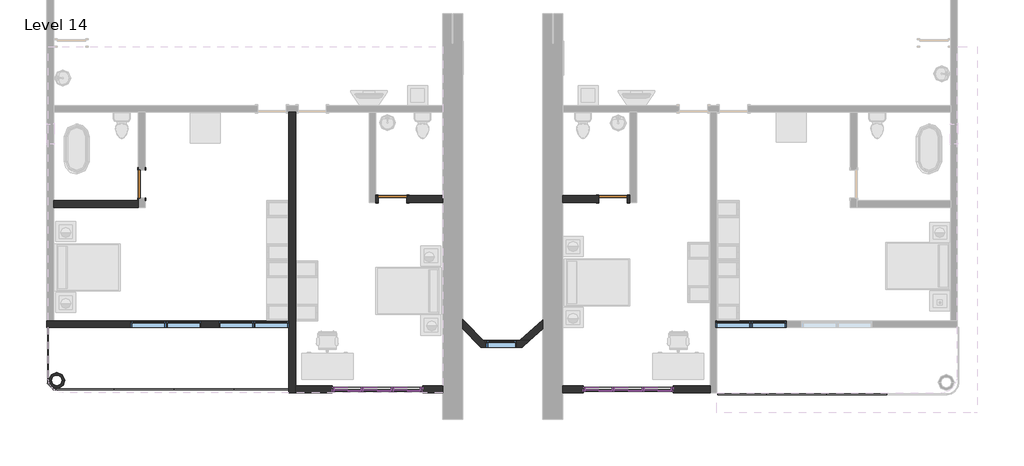
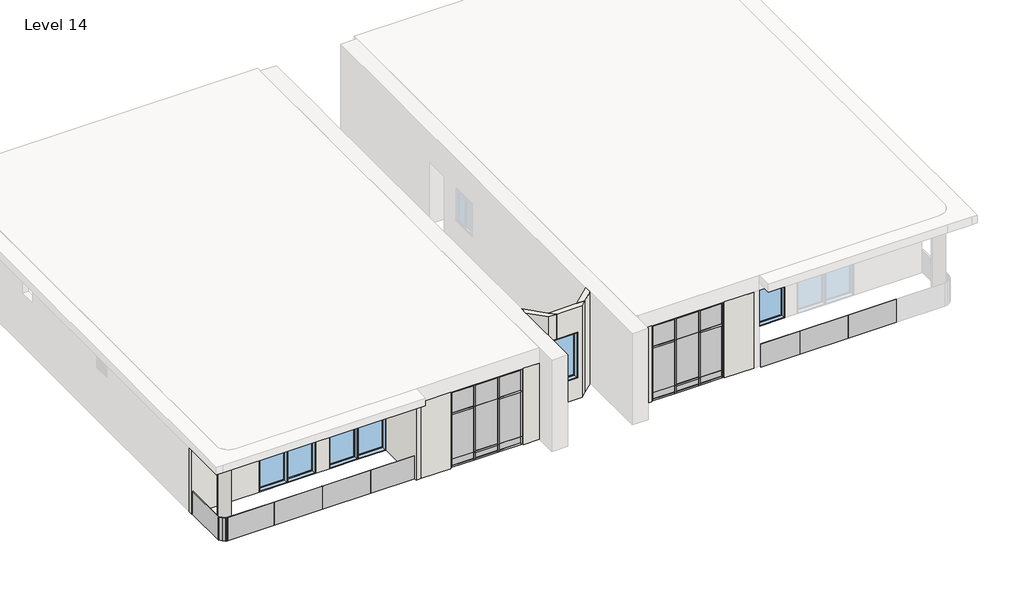
# One storey, part 1 of 3: 42 members, 30 plates, 14 walls, 7 windows, 3 doors.
"""IFC4 building model written with IfcOpenShell, lengths in millimetres."""

from ifc_helpers import new_model, si_unit, point, frame, frame_2d, origin, place, context, project, spatial, polyline, circle_curve, trimmed, segment, composite_curve, outline, extrude, faceted_brep, transform, mapped, element, save
from components import door_2703ae13, door_10fd3a06, member_c17f1be2, member_ad567e07, member_d2e7e466, member_7db1855a, member_75d1e245, member_d60e8053, member_3c3dc66a, member_2fae0574, member_410c6227, member_73c23c35, system_panel_glazed_38d54ecf, system_panel_glazed_fbb6c980, system_panel_glazed_4137532c, system_panel_glazed_6230de04, system_panel_glazed_a79f7f85, system_panel_glazed_9a5ea490, system_panel_glazed_95be5de7, system_panel_glazed_1e00a1c5, system_panel_glazed_ffe51582, system_panel_glazed_8f95e3f6, system_panel_glazed_836907cd, system_panel_glazed_688a65a2, system_panel_glazed_c1a1c740, system_panel_glazed_22bcd51f, window_9a779fa2, window_1a213a25

model = new_model("IFC4")

# Units and contexts
model_context = context("Model", 3, world=origin())
ifc_project = project(units=[si_unit("LENGTHUNIT", "METRE", prefix="MILLI")], contexts=[model_context])

# Site, building, storey
site = spatial("IfcSite", under=ifc_project)
building = spatial("IfcBuilding", under=site)
storey = spatial("IfcBuildingStorey", under=building, Name="Level 14", Elevation=47548.8)

# Doors
placement = place(None, origin())
door_shape = door_2703ae13(model_context)
element("IfcDoor", 1, ObjectType="Door-Single-Panel.0001 : 34\" x 80\"", at=placement, inside=storey, context=model_context, shape_type="MappedRepresentation", body=[
    mapped(door_shape, transform((-15765.9987704, -441.9241442, 47548.8), x_axis=(0.0, -1.0, 0.0), y_axis=(1.0, 0.0, 0.0), z_axis=(0.0, 0.0, 1.0))),
])
element("IfcDoor", 2, ObjectType="Door-Single-Panel.0001 : 34\" x 80\"", at=placement, inside=storey, context=model_context, shape_type="MappedRepresentation", body=[
    mapped(door_shape, transform((-8145.9987704, -899.1241442, 47548.8), x_axis=(-1.0, 0.0, 0.0), y_axis=(0.0, -1.0, 0.0), z_axis=(0.0, 0.0, 1.0))),
])
door_2_shape = door_10fd3a06(model_context)
element("IfcDoor", 3, ObjectType="Door-Single-Panel.0001 : 34\" x 80\"", at=placement, inside=storey, context=model_context, shape_type="MappedRepresentation", body=[
    mapped(door_2_shape, transform((-1440.3987704, -899.1241442, 47548.8), x_axis=(1.0, 0.0, 0.0), y_axis=(0.0, 1.0, 0.0), z_axis=(0.0, 0.0, 1.0))),
])

# Members
member_shape = member_c17f1be2(model_context)
element("IfcMember", 4, ObjectType="Rectangular Mullion : 2.5\" x 5\" rectangular", at=placement, inside=storey, context=model_context, shape_type="MappedRepresentation", body=[
    mapped(member_shape, transform((-9911.2987704, -6690.3241442, 50596.8), x_axis=(0.0, 0.0, 1.0), y_axis=(0.0, 1.0, 0.0), z_axis=(-1.0, 0.0, 0.0))),
])
element("IfcMember", 5, ObjectType="Rectangular Mullion : 2.5\" x 5\" rectangular", at=placement, inside=storey, context=model_context, shape_type="MappedRepresentation", body=[
    mapped(member_shape, transform((-8114.2487704, -6690.3241442, 50596.8), x_axis=(0.0, 0.0, 1.0), y_axis=(0.0, 1.0, 0.0), z_axis=(-1.0, 0.0, 0.0))),
])
element("IfcMember", 6, ObjectType="Rectangular Mullion : 2.5\" x 5\" rectangular", at=placement, inside=storey, context=model_context, shape_type="MappedRepresentation", body=[
    mapped(member_shape, transform((-2291.2987704, -6690.3241442, 50596.8), x_axis=(0.0, 0.0, 1.0), y_axis=(0.0, 1.0, 0.0), z_axis=(-1.0, 0.0, 0.0))),
])
element("IfcMember", 7, ObjectType="Rectangular Mullion : 2.5\" x 5\" rectangular", at=placement, inside=storey, context=model_context, shape_type="MappedRepresentation", body=[
    mapped(member_shape, transform((-494.2487704, -6690.3241442, 50596.8), x_axis=(0.0, 0.0, 1.0), y_axis=(0.0, 1.0, 0.0), z_axis=(-1.0, 0.0, 0.0))),
])
element("IfcMember", 8, ObjectType="Rectangular Mullion : 2.5\" x 5\" rectangular", at=placement, inside=storey, context=model_context, shape_type="MappedRepresentation", body=[
    mapped(member_shape, transform((-7295.0987704, -6690.3241442, 47548.8), x_axis=(0.0, 0.0, -1.0), y_axis=(0.0, 1.0, 0.0), z_axis=(1.0, 0.0, 0.0))),
])
element("IfcMember", 9, ObjectType="Rectangular Mullion : 2.5\" x 5\" rectangular", at=placement, inside=storey, context=model_context, shape_type="MappedRepresentation", body=[
    mapped(member_shape, transform((-9092.1487704, -6690.3241442, 47548.8), x_axis=(0.0, 0.0, -1.0), y_axis=(0.0, 1.0, 0.0), z_axis=(1.0, 0.0, 0.0))),
])
element("IfcMember", 10, ObjectType="Rectangular Mullion : 2.5\" x 5\" rectangular", at=placement, inside=storey, context=model_context, shape_type="MappedRepresentation", body=[
    mapped(member_shape, transform((324.9012296, -6690.3241442, 47548.8), x_axis=(0.0, 0.0, -1.0), y_axis=(0.0, 1.0, 0.0), z_axis=(1.0, 0.0, 0.0))),
])
element("IfcMember", 11, ObjectType="Rectangular Mullion : 2.5\" x 5\" rectangular", at=placement, inside=storey, context=model_context, shape_type="MappedRepresentation", body=[
    mapped(member_shape, transform((-1472.1487704, -6690.3241442, 47548.8), x_axis=(0.0, 0.0, -1.0), y_axis=(0.0, 1.0, 0.0), z_axis=(1.0, 0.0, 0.0))),
])
member_2_shape = member_ad567e07(model_context)
element("IfcMember", 12, ObjectType="Rectangular Mullion : 2.5\" x 5\" rectangular", at=placement, inside=storey, context=model_context, shape_type="MappedRepresentation", body=[
    mapped(member_2_shape, transform((-8114.2487704, -6690.3241442, 49682.4), x_axis=(0.0, 0.0, 1.0), y_axis=(0.0, 1.0, 0.0), z_axis=(-1.0, 0.0, 0.0))),
])
element("IfcMember", 13, ObjectType="Rectangular Mullion : 2.5\" x 5\" rectangular", at=placement, inside=storey, context=model_context, shape_type="MappedRepresentation", body=[
    mapped(member_2_shape, transform((-9911.2987704, -6690.3241442, 49682.4), x_axis=(0.0, 0.0, 1.0), y_axis=(0.0, 1.0, 0.0), z_axis=(-1.0, 0.0, 0.0))),
])
element("IfcMember", 14, ObjectType="Rectangular Mullion : 2.5\" x 5\" rectangular", at=placement, inside=storey, context=model_context, shape_type="MappedRepresentation", body=[
    mapped(member_2_shape, transform((-494.2487704, -6690.3241442, 49682.4), x_axis=(0.0, 0.0, 1.0), y_axis=(0.0, 1.0, 0.0), z_axis=(-1.0, 0.0, 0.0))),
])
element("IfcMember", 15, ObjectType="Rectangular Mullion : 2.5\" x 5\" rectangular", at=placement, inside=storey, context=model_context, shape_type="MappedRepresentation", body=[
    mapped(member_2_shape, transform((-2291.2987704, -6690.3241442, 49682.4), x_axis=(0.0, 0.0, 1.0), y_axis=(0.0, 1.0, 0.0), z_axis=(-1.0, 0.0, 0.0))),
])
member_3_shape = member_d2e7e466(model_context)
element("IfcMember", 16, ObjectType="Rectangular Mullion : 2.5\" x 5\" rectangular", at=placement, inside=storey, context=model_context, shape_type="MappedRepresentation", body=[
    mapped(member_3_shape, transform((-8177.7487704, -6690.3241442, 47548.8), x_axis=(0.0, 0.0, -1.0), y_axis=(0.0, 1.0, 0.0), z_axis=(1.0, 0.0, 0.0))),
])
element("IfcMember", 17, ObjectType="Rectangular Mullion : 2.5\" x 5\" rectangular", at=placement, inside=storey, context=model_context, shape_type="MappedRepresentation", body=[
    mapped(member_3_shape, transform((-557.7487704, -6690.3241442, 47548.8), x_axis=(0.0, 0.0, -1.0), y_axis=(0.0, 1.0, 0.0), z_axis=(1.0, 0.0, 0.0))),
])
member_4_shape = member_7db1855a(model_context)
element("IfcMember", 18, ObjectType="Rectangular Mullion : 2.5\" x 5\" rectangular", at=placement, inside=storey, context=model_context, shape_type="MappedRepresentation", body=[
    mapped(member_4_shape, transform((-9028.6487704, -6690.3241442, 47853.6), x_axis=(0.0, 0.0, 1.0), y_axis=(0.0, 1.0, 0.0), z_axis=(-1.0, 0.0, 0.0))),
])
element("IfcMember", 19, ObjectType="Rectangular Mullion : 2.5\" x 5\" rectangular", at=placement, inside=storey, context=model_context, shape_type="MappedRepresentation", body=[
    mapped(member_4_shape, transform((-1408.6487704, -6690.3241442, 47853.6), x_axis=(0.0, 0.0, 1.0), y_axis=(0.0, 1.0, 0.0), z_axis=(-1.0, 0.0, 0.0))),
])
element("IfcMember", 20, ObjectType="Rectangular Mullion : 2.5\" x 5\" rectangular", at=placement, inside=storey, context=model_context, shape_type="MappedRepresentation", body=[
    mapped(member_3_shape, transform((-9028.6487704, -6690.3241442, 50596.8), x_axis=(0.0, 0.0, 1.0), y_axis=(0.0, 1.0, 0.0), z_axis=(-1.0, 0.0, 0.0))),
])
element("IfcMember", 21, ObjectType="Rectangular Mullion : 2.5\" x 5\" rectangular", at=placement, inside=storey, context=model_context, shape_type="MappedRepresentation", body=[
    mapped(member_3_shape, transform((-1408.6487704, -6690.3241442, 50596.8), x_axis=(0.0, 0.0, 1.0), y_axis=(0.0, 1.0, 0.0), z_axis=(-1.0, 0.0, 0.0))),
])
member_5_shape = member_75d1e245(model_context)
element("IfcMember", 22, ObjectType="Rectangular Mullion : 2.5\" x 5\" rectangular", at=placement, inside=storey, context=model_context, shape_type="MappedRepresentation", body=[
    mapped(member_5_shape, transform((-8145.9987704, -6690.3241442, 47548.8), x_axis=(-1.0, 0.0, 0.0), y_axis=(0.0, 1.0, 0.0), z_axis=(0.0, 0.0, -1.0))),
])
element("IfcMember", 23, ObjectType="Rectangular Mullion : 2.5\" x 5\" rectangular", at=placement, inside=storey, context=model_context, shape_type="MappedRepresentation", body=[
    mapped(member_5_shape, transform((-9060.3987704, -6690.3241442, 47548.8), x_axis=(-1.0, 0.0, 0.0), y_axis=(0.0, 1.0, 0.0), z_axis=(0.0, 0.0, -1.0))),
])
element("IfcMember", 24, ObjectType="Rectangular Mullion : 2.5\" x 5\" rectangular", at=placement, inside=storey, context=model_context, shape_type="MappedRepresentation", body=[
    mapped(member_5_shape, transform((-525.9987704, -6690.3241442, 47548.8), x_axis=(-1.0, 0.0, 0.0), y_axis=(0.0, 1.0, 0.0), z_axis=(0.0, 0.0, -1.0))),
])
element("IfcMember", 25, ObjectType="Rectangular Mullion : 2.5\" x 5\" rectangular", at=placement, inside=storey, context=model_context, shape_type="MappedRepresentation", body=[
    mapped(member_5_shape, transform((-1440.3987704, -6690.3241442, 47548.8), x_axis=(-1.0, 0.0, 0.0), y_axis=(0.0, 1.0, 0.0), z_axis=(0.0, 0.0, -1.0))),
])
member_6_shape = member_d60e8053(model_context)
element("IfcMember", 26, ObjectType="Rectangular Mullion : 2.5\" x 5\" rectangular", at=placement, inside=storey, context=model_context, shape_type="MappedRepresentation", body=[
    mapped(member_6_shape, transform((-8145.9987704, -6690.3241442, 47853.6), x_axis=(-1.0, 0.0, 0.0), y_axis=(0.0, 1.0, 0.0), z_axis=(0.0, 0.0, -1.0))),
])
element("IfcMember", 27, ObjectType="Rectangular Mullion : 2.5\" x 5\" rectangular", at=placement, inside=storey, context=model_context, shape_type="MappedRepresentation", body=[
    mapped(member_6_shape, transform((-9060.3987704, -6690.3241442, 47853.6), x_axis=(-1.0, 0.0, 0.0), y_axis=(0.0, 1.0, 0.0), z_axis=(0.0, 0.0, -1.0))),
])
element("IfcMember", 28, ObjectType="Rectangular Mullion : 2.5\" x 5\" rectangular", at=placement, inside=storey, context=model_context, shape_type="MappedRepresentation", body=[
    mapped(member_6_shape, transform((-525.9987704, -6690.3241442, 47853.6), x_axis=(-1.0, 0.0, 0.0), y_axis=(0.0, 1.0, 0.0), z_axis=(0.0, 0.0, -1.0))),
])
element("IfcMember", 29, ObjectType="Rectangular Mullion : 2.5\" x 5\" rectangular", at=placement, inside=storey, context=model_context, shape_type="MappedRepresentation", body=[
    mapped(member_6_shape, transform((-1440.3987704, -6690.3241442, 47853.6), x_axis=(-1.0, 0.0, 0.0), y_axis=(0.0, 1.0, 0.0), z_axis=(0.0, 0.0, -1.0))),
])
member_7_shape = member_3c3dc66a(model_context)
element("IfcMember", 30, ObjectType="Rectangular Mullion : 2.5\" x 5\" rectangular", at=placement, inside=storey, context=model_context, shape_type="MappedRepresentation", body=[
    mapped(member_7_shape, transform((-9974.7987704, -6690.3241442, 47548.8), x_axis=(-1.0, 0.0, 0.0), y_axis=(0.0, 1.0, 0.0), z_axis=(0.0, 0.0, -1.0))),
])
element("IfcMember", 31, ObjectType="Rectangular Mullion : 2.5\" x 5\" rectangular", at=placement, inside=storey, context=model_context, shape_type="MappedRepresentation", body=[
    mapped(member_7_shape, transform((-2354.7987704, -6690.3241442, 47548.8), x_axis=(-1.0, 0.0, 0.0), y_axis=(0.0, 1.0, 0.0), z_axis=(0.0, 0.0, -1.0))),
])
member_8_shape = member_2fae0574(model_context)
element("IfcMember", 32, ObjectType="Rectangular Mullion : 2.5\" x 5\" rectangular", at=placement, inside=storey, context=model_context, shape_type="MappedRepresentation", body=[
    mapped(member_8_shape, transform((-9974.7987704, -6690.3241442, 47853.6), x_axis=(-1.0, 0.0, 0.0), y_axis=(0.0, 1.0, 0.0), z_axis=(0.0, 0.0, -1.0))),
])
element("IfcMember", 33, ObjectType="Rectangular Mullion : 2.5\" x 5\" rectangular", at=placement, inside=storey, context=model_context, shape_type="MappedRepresentation", body=[
    mapped(member_8_shape, transform((-2354.7987704, -6690.3241442, 47853.6), x_axis=(-1.0, 0.0, 0.0), y_axis=(0.0, 1.0, 0.0), z_axis=(0.0, 0.0, -1.0))),
])
element("IfcMember", 34, ObjectType="Rectangular Mullion : 2.5\" x 5\" rectangular", at=placement, inside=storey, context=model_context, shape_type="MappedRepresentation", body=[
    mapped(member_8_shape, transform((-7231.5987704, -6690.3241442, 49682.4), x_axis=(1.0, 0.0, 0.0), y_axis=(0.0, 1.0, 0.0), z_axis=(0.0, 0.0, 1.0))),
])
element("IfcMember", 35, ObjectType="Rectangular Mullion : 2.5\" x 5\" rectangular", at=placement, inside=storey, context=model_context, shape_type="MappedRepresentation", body=[
    mapped(member_8_shape, transform((388.4012296, -6690.3241442, 49682.4), x_axis=(1.0, 0.0, 0.0), y_axis=(0.0, 1.0, 0.0), z_axis=(0.0, 0.0, 1.0))),
])
element("IfcMember", 36, ObjectType="Rectangular Mullion : 2.5\" x 5\" rectangular", at=placement, inside=storey, context=model_context, shape_type="MappedRepresentation", body=[
    mapped(member_7_shape, transform((-7231.5987704, -6690.3241442, 47853.6), x_axis=(1.0, 0.0, 0.0), y_axis=(0.0, 1.0, 0.0), z_axis=(0.0, 0.0, 1.0))),
])
element("IfcMember", 37, ObjectType="Rectangular Mullion : 2.5\" x 5\" rectangular", at=placement, inside=storey, context=model_context, shape_type="MappedRepresentation", body=[
    mapped(member_7_shape, transform((388.4012296, -6690.3241442, 47853.6), x_axis=(1.0, 0.0, 0.0), y_axis=(0.0, 1.0, 0.0), z_axis=(0.0, 0.0, 1.0))),
])
member_9_shape = member_410c6227(model_context)
element("IfcMember", 38, ObjectType="Rectangular Mullion : 2.5\" x 5\" rectangular", at=placement, inside=storey, context=model_context, shape_type="MappedRepresentation", body=[
    mapped(member_9_shape, transform((-8145.9987704, -6690.3241442, 49682.4), x_axis=(-1.0, 0.0, 0.0), y_axis=(0.0, 1.0, 0.0), z_axis=(0.0, 0.0, -1.0))),
])
element("IfcMember", 39, ObjectType="Rectangular Mullion : 2.5\" x 5\" rectangular", at=placement, inside=storey, context=model_context, shape_type="MappedRepresentation", body=[
    mapped(member_9_shape, transform((-9060.3987704, -6690.3241442, 49682.4), x_axis=(-1.0, 0.0, 0.0), y_axis=(0.0, 1.0, 0.0), z_axis=(0.0, 0.0, -1.0))),
])
element("IfcMember", 40, ObjectType="Rectangular Mullion : 2.5\" x 5\" rectangular", at=placement, inside=storey, context=model_context, shape_type="MappedRepresentation", body=[
    mapped(member_9_shape, transform((-525.9987704, -6690.3241442, 49682.4), x_axis=(-1.0, 0.0, 0.0), y_axis=(0.0, 1.0, 0.0), z_axis=(0.0, 0.0, -1.0))),
])
element("IfcMember", 41, ObjectType="Rectangular Mullion : 2.5\" x 5\" rectangular", at=placement, inside=storey, context=model_context, shape_type="MappedRepresentation", body=[
    mapped(member_9_shape, transform((-1440.3987704, -6690.3241442, 49682.4), x_axis=(-1.0, 0.0, 0.0), y_axis=(0.0, 1.0, 0.0), z_axis=(0.0, 0.0, -1.0))),
])
member_10_shape = member_73c23c35(model_context)
element("IfcMember", 42, ObjectType="Rectangular Mullion : 2.5\" x 5\" rectangular", at=placement, inside=storey, context=model_context, shape_type="MappedRepresentation", body=[
    mapped(member_10_shape, transform((-7231.5987704, -6690.3241442, 50596.8), x_axis=(1.0, 0.0, 0.0), y_axis=(0.0, 1.0, 0.0), z_axis=(0.0, 0.0, 1.0))),
])
element("IfcMember", 43, ObjectType="Rectangular Mullion : 2.5\" x 5\" rectangular", at=placement, inside=storey, context=model_context, shape_type="MappedRepresentation", body=[
    mapped(member_10_shape, transform((388.4012296, -6690.3241442, 50596.8), x_axis=(1.0, 0.0, 0.0), y_axis=(0.0, 1.0, 0.0), z_axis=(0.0, 0.0, 1.0))),
])
element("IfcMember", 44, ObjectType="Rectangular Mullion : 2.5\" x 5\" rectangular", at=placement, inside=storey, context=model_context, shape_type="MappedRepresentation", body=[
    mapped(member_10_shape, transform((-9974.7987704, -6690.3241442, 49682.4), x_axis=(-1.0, 0.0, 0.0), y_axis=(0.0, 1.0, 0.0), z_axis=(0.0, 0.0, -1.0))),
])
element("IfcMember", 45, ObjectType="Rectangular Mullion : 2.5\" x 5\" rectangular", at=placement, inside=storey, context=model_context, shape_type="MappedRepresentation", body=[
    mapped(member_10_shape, transform((-2354.7987704, -6690.3241442, 49682.4), x_axis=(-1.0, 0.0, 0.0), y_axis=(0.0, 1.0, 0.0), z_axis=(0.0, 0.0, -1.0))),
])

# Plates
system_panel_glazed_shape = system_panel_glazed_38d54ecf(model_context)
element("IfcPlate", 46, ObjectType="System Panel : Glazed", at=placement, inside=storey, context=model_context, shape_type="MappedRepresentation", body=[
    mapped(system_panel_glazed_shape, transform((-8603.1987704, -6690.3241442, 47885.35), x_axis=(-1.0, 0.0, 0.0), y_axis=(0.0, -1.0, 0.0), z_axis=(0.0, 0.0, 1.0))),
])
element("IfcPlate", 47, ObjectType="System Panel : Glazed", at=placement, inside=storey, context=model_context, shape_type="MappedRepresentation", body=[
    mapped(system_panel_glazed_shape, transform((-983.1987704, -6690.3241442, 47885.35), x_axis=(-1.0, 0.0, 0.0), y_axis=(0.0, -1.0, 0.0), z_axis=(0.0, 0.0, 1.0))),
])
system_panel_glazed_2_shape = system_panel_glazed_fbb6c980(model_context)
element("IfcPlate", 48, ObjectType="System Panel : Glazed", at=placement, inside=storey, context=model_context, shape_type="MappedRepresentation", body=[
    mapped(system_panel_glazed_2_shape, transform((-8603.1987704, -6690.3241442, 47612.3), x_axis=(-1.0, 0.0, 0.0), y_axis=(0.0, -1.0, 0.0), z_axis=(0.0, 0.0, 1.0))),
])
element("IfcPlate", 49, ObjectType="System Panel : Glazed", at=placement, inside=storey, context=model_context, shape_type="MappedRepresentation", body=[
    mapped(system_panel_glazed_2_shape, transform((-983.1987704, -6690.3241442, 47612.3), x_axis=(-1.0, 0.0, 0.0), y_axis=(0.0, -1.0, 0.0), z_axis=(0.0, 0.0, 1.0))),
])
system_panel_glazed_3_shape = system_panel_glazed_4137532c(model_context)
element("IfcPlate", 50, ObjectType="System Panel : Glazed", at=placement, inside=storey, context=model_context, shape_type="MappedRepresentation", body=[
    mapped(system_panel_glazed_3_shape, transform((-7704.6737704, -6690.3241442, 47612.3), x_axis=(-1.0, 0.0, 0.0), y_axis=(0.0, -1.0, 0.0), z_axis=(0.0, 0.0, 1.0))),
])
element("IfcPlate", 51, ObjectType="System Panel : Glazed", at=placement, inside=storey, context=model_context, shape_type="MappedRepresentation", body=[
    mapped(system_panel_glazed_3_shape, transform((-9501.7237704, -6690.3241442, 47612.3), x_axis=(-1.0, 0.0, 0.0), y_axis=(0.0, -1.0, 0.0), z_axis=(0.0, 0.0, 1.0))),
])
element("IfcPlate", 52, ObjectType="System Panel : Glazed", at=placement, inside=storey, context=model_context, shape_type="MappedRepresentation", body=[
    mapped(system_panel_glazed_3_shape, transform((-84.6737704, -6690.3241442, 47612.3), x_axis=(-1.0, 0.0, 0.0), y_axis=(0.0, -1.0, 0.0), z_axis=(0.0, 0.0, 1.0))),
])
element("IfcPlate", 53, ObjectType="System Panel : Glazed", at=placement, inside=storey, context=model_context, shape_type="MappedRepresentation", body=[
    mapped(system_panel_glazed_3_shape, transform((-1881.7237704, -6690.3241442, 47612.3), x_axis=(-1.0, 0.0, 0.0), y_axis=(0.0, -1.0, 0.0), z_axis=(0.0, 0.0, 1.0))),
])
system_panel_glazed_4_shape = system_panel_glazed_6230de04(model_context)
element("IfcPlate", 54, ObjectType="System Panel : Glazed", at=placement, inside=storey, context=model_context, shape_type="MappedRepresentation", body=[
    mapped(system_panel_glazed_4_shape, transform((-7704.6737704, -6690.3241442, 47853.6), x_axis=(-1.0, 0.0, 0.0), y_axis=(0.0, -1.0, 0.0), z_axis=(0.0, 0.0, 1.0))),
])
element("IfcPlate", 55, ObjectType="System Panel : Glazed", at=placement, inside=storey, context=model_context, shape_type="MappedRepresentation", body=[
    mapped(system_panel_glazed_4_shape, transform((-9501.7237704, -6690.3241442, 47853.6), x_axis=(-1.0, 0.0, 0.0), y_axis=(0.0, -1.0, 0.0), z_axis=(0.0, 0.0, 1.0))),
])
element("IfcPlate", 56, ObjectType="System Panel : Glazed", at=placement, inside=storey, context=model_context, shape_type="MappedRepresentation", body=[
    mapped(system_panel_glazed_4_shape, transform((-84.6737704, -6690.3241442, 47853.6), x_axis=(-1.0, 0.0, 0.0), y_axis=(0.0, -1.0, 0.0), z_axis=(0.0, 0.0, 1.0))),
])
element("IfcPlate", 57, ObjectType="System Panel : Glazed", at=placement, inside=storey, context=model_context, shape_type="MappedRepresentation", body=[
    mapped(system_panel_glazed_4_shape, transform((-1881.7237704, -6690.3241442, 47853.6), x_axis=(-1.0, 0.0, 0.0), y_axis=(0.0, -1.0, 0.0), z_axis=(0.0, 0.0, 1.0))),
])
system_panel_glazed_5_shape = system_panel_glazed_a79f7f85(model_context)
element("IfcPlate", 58, ObjectType="System Panel : Glazed", at=placement, inside=storey, context=model_context, shape_type="MappedRepresentation", body=[
    mapped(system_panel_glazed_5_shape, transform((-7704.6737704, -6690.3241442, 49714.15), x_axis=(-1.0, 0.0, 0.0), y_axis=(0.0, -1.0, 0.0), z_axis=(0.0, 0.0, 1.0))),
])
element("IfcPlate", 59, ObjectType="System Panel : Glazed", at=placement, inside=storey, context=model_context, shape_type="MappedRepresentation", body=[
    mapped(system_panel_glazed_5_shape, transform((-9501.7237704, -6690.3241442, 49714.15), x_axis=(-1.0, 0.0, 0.0), y_axis=(0.0, -1.0, 0.0), z_axis=(0.0, 0.0, 1.0))),
])
element("IfcPlate", 60, ObjectType="System Panel : Glazed", at=placement, inside=storey, context=model_context, shape_type="MappedRepresentation", body=[
    mapped(system_panel_glazed_5_shape, transform((-84.6737704, -6690.3241442, 49714.15), x_axis=(-1.0, 0.0, 0.0), y_axis=(0.0, -1.0, 0.0), z_axis=(0.0, 0.0, 1.0))),
])
element("IfcPlate", 61, ObjectType="System Panel : Glazed", at=placement, inside=storey, context=model_context, shape_type="MappedRepresentation", body=[
    mapped(system_panel_glazed_5_shape, transform((-1881.7237704, -6690.3241442, 49714.15), x_axis=(-1.0, 0.0, 0.0), y_axis=(0.0, -1.0, 0.0), z_axis=(0.0, 0.0, 1.0))),
])
system_panel_glazed_6_shape = system_panel_glazed_9a5ea490(model_context)
element("IfcPlate", 62, ObjectType="System Panel : Glazed", at=placement, inside=storey, context=model_context, shape_type="MappedRepresentation", body=[
    mapped(system_panel_glazed_6_shape, transform((-8603.1987704, -6690.3241442, 49682.4), x_axis=(-1.0, 0.0, 0.0), y_axis=(0.0, -1.0, 0.0), z_axis=(0.0, 0.0, 1.0))),
])
element("IfcPlate", 63, ObjectType="System Panel : Glazed", at=placement, inside=storey, context=model_context, shape_type="MappedRepresentation", body=[
    mapped(system_panel_glazed_6_shape, transform((-983.1987704, -6690.3241442, 49682.4), x_axis=(-1.0, 0.0, 0.0), y_axis=(0.0, -1.0, 0.0), z_axis=(0.0, 0.0, 1.0))),
])
system_panel_glazed_7_shape = system_panel_glazed_95be5de7(model_context)
element("IfcPlate", 64, ObjectType="System Panel : Glazed", at=placement, inside=storey, context=model_context, shape_type="MappedRepresentation", body=[
    mapped(system_panel_glazed_7_shape, transform((-15707.2305745, -6723.6923401, 47548.8), x_axis=(1.0, 0.0, 0.0), y_axis=(0.0, 1.0, 0.0), z_axis=(0.0, 0.0, 1.0))),
])
element("IfcPlate", 65, ObjectType="System Panel : Glazed", at=placement, inside=storey, context=model_context, shape_type="MappedRepresentation", body=[
    mapped(system_panel_glazed_7_shape, transform((-13878.4305745, -6723.6923401, 47548.8), x_axis=(1.0, 0.0, 0.0), y_axis=(0.0, 1.0, 0.0), z_axis=(0.0, 0.0, 1.0))),
])
element("IfcPlate", 66, ObjectType="System Panel : Glazed", at=placement, inside=storey, context=model_context, shape_type="MappedRepresentation", body=[
    mapped(system_panel_glazed_7_shape, transform((5957.9120092, -6810.4133646, 47548.8), x_axis=(-1.0, 0.0, 0.0), y_axis=(0.0, -1.0, 0.0), z_axis=(0.0, 0.0, 1.0))),
])
element("IfcPlate", 67, ObjectType="System Panel : Glazed", at=placement, inside=storey, context=model_context, shape_type="MappedRepresentation", body=[
    mapped(system_panel_glazed_7_shape, transform((4129.1120092, -6810.4133646, 47548.8), x_axis=(-1.0, 0.0, 0.0), y_axis=(0.0, -1.0, 0.0), z_axis=(0.0, 0.0, 1.0))),
])
system_panel_glazed_8_shape = system_panel_glazed_1e00a1c5(model_context)
element("IfcPlate", 68, ObjectType="System Panel : Glazed", at=placement, inside=storey, context=model_context, shape_type="MappedRepresentation", body=[
    mapped(system_panel_glazed_8_shape, transform((2478.1120092, -6810.4133646, 47548.8), x_axis=(-1.0, 0.0, 0.0), y_axis=(0.0, -1.0, 0.0), z_axis=(0.0, 0.0, 1.0))),
])
system_panel_glazed_9_shape = system_panel_glazed_ffe51582(model_context)
element("IfcPlate", 69, ObjectType="System Panel : Glazed", at=placement, inside=storey, context=model_context, shape_type="MappedRepresentation", body=[
    mapped(system_panel_glazed_9_shape, transform((-18451.9713429, -6722.1515718, 47548.8), x_axis=(0.7071067811865462, -0.7071067811865488, 0.0), y_axis=(0.7071067811865488, 0.7071067811865462, 0.0), z_axis=(0.0, 0.0, 1.0))),
])
system_panel_glazed_10_shape = system_panel_glazed_8f95e3f6(model_context)
element("IfcPlate", 70, ObjectType="System Panel : Glazed", at=placement, inside=storey, context=model_context, shape_type="MappedRepresentation", body=[
    mapped(system_panel_glazed_10_shape, transform((-18648.8987704, -5667.9741442, 47548.8), x_axis=(0.0, -1.0, 0.0), y_axis=(1.0, 0.0, 0.0), z_axis=(0.0, 0.0, 1.0))),
])
system_panel_glazed_11_shape = system_panel_glazed_836907cd(model_context)
element("IfcPlate", 71, ObjectType="System Panel : Glazed", at=placement, inside=storey, context=model_context, shape_type="MappedRepresentation", body=[
    mapped(system_panel_glazed_11_shape, transform((-18418.6805745, -6723.6923401, 47548.8), x_axis=(1.0, 0.0, 0.0), y_axis=(0.0, 1.0, 0.0), z_axis=(0.0, 0.0, 1.0))),
])
system_panel_glazed_12_shape = system_panel_glazed_688a65a2(model_context)
element("IfcPlate", 72, ObjectType="System Panel : Glazed", at=placement, inside=storey, context=model_context, shape_type="MappedRepresentation", body=[
    mapped(system_panel_glazed_12_shape, transform((-12129.8146725, -6723.6923401, 47548.8), x_axis=(1.0, 0.0, 0.0), y_axis=(0.0, 1.0, 0.0), z_axis=(0.0, 0.0, 1.0))),
])
system_panel_glazed_13_shape = system_panel_glazed_c1a1c740(model_context)
element("IfcPlate", 73, ObjectType="System Panel : Glazed", at=placement, inside=storey, context=model_context, shape_type="MappedRepresentation", body=[
    mapped(system_panel_glazed_13_shape, transform((-17504.2805745, -6723.6923401, 47548.8), x_axis=(1.0, 0.0, 0.0), y_axis=(0.0, 1.0, 0.0), z_axis=(0.0, 0.0, 1.0))),
])
system_panel_glazed_14_shape = system_panel_glazed_22bcd51f(model_context)
element("IfcPlate", 74, ObjectType="System Panel : Glazed", at=placement, inside=storey, context=model_context, shape_type="MappedRepresentation", body=[
    mapped(system_panel_glazed_14_shape, transform((-18600.0521056, -6574.070809, 47548.8), x_axis=(0.7071067811865462, -0.7071067811865488, 0.0), y_axis=(0.7071067811865488, 0.7071067811865462, 0.0), z_axis=(0.0, 0.0, 1.0))),
])
element("IfcPlate", 75, ObjectType="System Panel : Glazed", at=placement, inside=storey, context=model_context, shape_type="MappedRepresentation", body=[
    mapped(system_panel_glazed_14_shape, transform((-18502.3587761, -6671.7641386, 47548.8), x_axis=(0.7071067811865462, -0.7071067811865488, 0.0), y_axis=(0.7071067811865488, 0.7071067811865462, 0.0), z_axis=(0.0, 0.0, 1.0))),
])

# Walls
element("IfcWall", 76, ObjectType="Generic - 3\" green 2", at=placement, inside=storey, context=model_context, shape_type="SweptSolid", body=[
    extrude(outline(composite_curve([segment(polyline([(-18518.7237704, -6418.8616442), (-18594.9237704, -6418.8616442)]), True, "CONTINUOUS"), segment(trimmed(circle_curve(frame_2d((-18353.6237704, -6418.8616442)), 241.3), [point((-18594.9237704, -6418.8616442))], [point((-18112.3237704, -6418.8616442))], False, "CARTESIAN"), True, "CONTINUOUS"), segment(polyline([(-18112.3237704, -6418.8616442), (-18188.5237704, -6418.8616442)]), True, "CONTINUOUS"), segment(trimmed(circle_curve(frame_2d((-18353.6237704, -6418.8616442)), 165.1), [point((-18188.5237704, -6418.8616442))], [point((-18518.7237704, -6418.8616442))], True, "CARTESIAN"), True, "CONTINUOUS")], self_intersect=False)), frame((0.0, 0.0, 47548.8), z_axis=(0.0, 0.0, 1.0), x_axis=(1.0, 0.0, 0.0)), (0.0, 0.0, 1.0), 3048.0),
])
element("IfcWall", 77, ObjectType="Generic - 3\" green 2", at=placement, inside=storey, context=model_context, shape_type="SweptSolid", body=[
    extrude(outline(composite_curve([segment(polyline([(-18188.5237704, -6418.8616442), (-18112.3237704, -6418.8616442)]), True, "CONTINUOUS"), segment(trimmed(circle_curve(frame_2d((-18353.6237704, -6418.8616442)), 241.3), [point((-18112.3237704, -6418.8616442))], [point((-18594.9237704, -6418.8616442))], False, "CARTESIAN"), True, "CONTINUOUS"), segment(polyline([(-18594.9237704, -6418.8616442), (-18518.7237704, -6418.8616442)]), True, "CONTINUOUS"), segment(trimmed(circle_curve(frame_2d((-18353.6237704, -6418.8616442)), 165.1), [point((-18518.7237704, -6418.8616442))], [point((-18188.5237704, -6418.8616442))], True, "CARTESIAN"), True, "CONTINUOUS")], self_intersect=False)), frame((0.0, 0.0, 47548.8), z_axis=(0.0, 0.0, 1.0), x_axis=(1.0, 0.0, 0.0)), (0.0, 0.0, 1.0), 3048.0),
])
element("IfcWall", 78, ObjectType="Generic - 8\" cream", at=placement, inside=storey, context=model_context, shape_type="Brep", body=[
    faceted_brep([(-11295.5987704, 1742.4758558, 47548.8), (-11295.5987704, -6791.9241442, 47548.8), (-11295.5987704, -6791.9241442, 50596.8), (-11295.5987704, -4810.7241442, 50596.8), (-11295.5987704, -4607.5241442, 50596.8), (-11295.5987704, 1742.4758558, 50596.8), (-11092.3987704, 1742.4758558, 47548.8), (-11092.3987704, 1742.4758558, 50596.8), (-11092.3987704, -6588.7241442, 50596.8), (-11092.3987704, -6791.9241442, 50596.8), (-11092.3987704, -6791.9241442, 47548.8), (-11092.3987704, -6588.7241442, 47548.8)], [[[0, 1, 2, 3, 4, 5]], [[6, 7, 8, 9, 10, 11]], [[1, 0, 6, 11, 10]], [[5, 4, 3, 2, 9, 8, 7]], [[0, 5, 7, 6]], [[2, 1, 10, 9]]]),
])
element("IfcWall", 79, ObjectType="Generic - 8\" cream", at=placement, inside=storey, context=model_context, shape_type="SweptSolid", body=[
    extrude(outline(polyline([(-18445.6987704, -949.9241442), (-15867.5987704, -949.9241442), (-15867.5987704, -1153.1241442), (-18445.6987704, -1153.1241442), (-18445.6987704, -949.9241442)])), frame((0.0, 0.0, 47548.8), z_axis=(0.0, 0.0, 1.0), x_axis=(1.0, 0.0, 0.0)), (0.0, 0.0, 1.0), 3048.0),
])
element("IfcWall", 80, ObjectType="Generic - 8\" cream", at=placement, inside=storey, context=model_context, shape_type="SweptSolid", body=[
    extrude(outline(polyline([(50596.8, -6621.9987704), (50596.8, -8653.9987704), (47548.8, -8653.9987704), (47548.8, -8577.7987704), (49580.8, -8577.7987704), (49580.8, -7714.1987704), (47548.8, -7714.1987704), (47548.8, -6621.9987704), (50596.8, -6621.9987704)])), frame((0.0, -1000.7241442, 0.0), z_axis=(0.0, 1.0, 0.0), x_axis=(0.0, 0.0, 1.0)), (0.0, 0.0, 1.0), 203.2),
])
element("IfcWall", 81, ObjectType="Generic - 8\" cream", at=placement, inside=storey, context=model_context, shape_type="Brep", body=[
    faceted_brep([(-18648.8987704, -4607.5241442, 50596.8), (-18445.6987704, -4607.5241442, 50596.8), (-11295.5987704, -4607.5241442, 50596.8), (-11295.5987704, -4607.5241442, 50292.0), (-13429.1987704, -4607.5241442, 50292.0), (-13429.1987704, -4607.5241442, 47548.8), (-13962.5987704, -4607.5241442, 47548.8), (-13962.5987704, -4607.5241442, 50292.0), (-16096.1987704, -4607.5241442, 50292.0), (-16096.1987704, -4607.5241442, 47548.8), (-18445.6987704, -4607.5241442, 47548.8), (-18648.8987704, -4607.5241442, 47548.8), (-11295.5987704, -4810.7241442, 50596.8), (-18648.8987704, -4810.7241442, 50596.8), (-18648.8987704, -4810.7241442, 47548.8), (-16096.1987704, -4810.7241442, 47548.8), (-16096.1987704, -4810.7241442, 50292.0), (-13962.5987704, -4810.7241442, 50292.0), (-13962.5987704, -4810.7241442, 47548.8), (-13429.1987704, -4810.7241442, 47548.8), (-13429.1987704, -4810.7241442, 50292.0), (-11295.5987704, -4810.7241442, 50292.0)], [[[0, 1, 2, 3, 4, 5, 6, 7, 8, 9, 10, 11]], [[12, 13, 14, 15, 16, 17, 18, 19, 20, 21]], [[14, 11, 10, 9, 15]], [[5, 19, 18, 6]], [[2, 1, 0, 13, 12]], [[2, 12, 21, 3]], [[0, 11, 14, 13]], [[3, 21, 20, 4]], [[4, 20, 19, 5]], [[17, 7, 6, 18]], [[7, 17, 16, 8]], [[8, 16, 15, 9]]]),
])
element("IfcWall", 82, ObjectType="Generic - 8\" cream", at=placement, inside=storey, context=model_context, shape_type="SweptSolid", body=[
    extrude(outline(polyline([(50596.8, -932.3987704), (50596.8, -2964.3987704), (47548.8, -2964.3987704), (47548.8, -1872.1987704), (49580.8, -1872.1987704), (49580.8, -1008.5987704), (47548.8, -1008.5987704), (47548.8, -932.3987704), (50596.8, -932.3987704)])), frame((0.0, -1000.7241442, 0.0), z_axis=(0.0, 1.0, 0.0), x_axis=(0.0, 0.0, 1.0)), (0.0, 0.0, 1.0), 203.2),
])
element("IfcWall", 83, ObjectType="Generic - 8\" green", at=placement, inside=storey, context=model_context, shape_type="Brep", body=[
    faceted_brep([(-6012.3987704, -4852.8082422, 47548.8), (-5458.7044276, -5406.502585, 47548.8), (-5458.7044276, -5406.502585, 51206.4), (-6012.3987704, -4852.8082422, 51206.4), (-5171.3362318, -5406.502585, 47548.8), (-5374.5362318, -5203.302585, 47548.8), (-6012.3987704, -4565.4400463, 47548.8), (-6012.3987704, -4565.4400463, 51206.4), (-5374.5362318, -5203.302585, 51206.4), (-5171.3362318, -5406.502585, 51206.4), (-5171.3362318, -5406.502585, 50215.8), (-5289.4901401, -5288.3486766, 50215.8), (-5289.4901401, -5288.3486766, 48387.0), (-5171.3362318, -5406.502585, 48387.0), (-5289.4901401, -5406.502585, 48387.0), (-5289.4901401, -5406.502585, 50215.8)], [[[0, 1, 2, 3]], [[4, 5, 6, 7, 8, 9, 10, 11, 12, 13]], [[1, 0, 6, 5, 4]], [[3, 2, 9, 8, 7]], [[0, 3, 7, 6]], [[2, 1, 4, 13, 14, 15, 10, 9]], [[12, 14, 13]], [[14, 12, 11, 15]], [[15, 11, 10]]]),
])
element("IfcWall", 84, ObjectType="Generic - 8\" green", at=placement, inside=storey, context=model_context, shape_type="Brep", body=[
    faceted_brep([(-5171.3362318, -5406.502585, 47548.8), (-4203.3343712, -5406.502585, 47548.8), (-4203.3343712, -5406.502585, 51206.4), (-5171.3362318, -5406.502585, 51206.4), (-5171.3362318, -5406.502585, 50215.8), (-4375.0901401, -5406.502585, 50215.8), (-4375.0901401, -5406.502585, 48387.0), (-5171.3362318, -5406.502585, 48387.0), (-3975.4820774, -5203.302585, 47548.8), (-4280.7801413, -5203.302585, 47548.8), (-5374.5362318, -5203.302585, 47548.8), (-5374.5362318, -5203.302585, 51206.4), (-4280.7801413, -5203.302585, 51206.4), (-3975.4820774, -5203.302585, 51206.4), (-4375.0901401, -5203.302585, 48387.0), (-4375.0901401, -5203.302585, 50215.8), (-5289.4901401, -5203.302585, 50215.8), (-5289.4901401, -5203.302585, 48387.0), (-5289.4901401, -5288.3486766, 48387.0), (-5289.4901401, -5288.3486766, 50215.8)], [[[0, 1, 2, 3, 4, 5, 6, 7]], [[8, 9, 10, 11, 12, 13], [14, 15, 16, 17]], [[1, 0, 10, 9, 8]], [[3, 2, 13, 12, 11]], [[3, 11, 10, 0, 7, 18, 19, 4]], [[2, 1, 8, 13]], [[5, 15, 14, 6]], [[6, 14, 17, 18, 7]], [[18, 17, 16, 19]], [[15, 5, 4, 19, 16]]]),
])
element("IfcWall", 85, ObjectType="Generic - 8\" green", at=placement, inside=storey, context=model_context, shape_type="SweptSolid", body=[
    extrude(outline(polyline([(-3573.9987704, -4845.2574382), (-3975.4820774, -5203.302585), (-4280.7801413, -5203.302585), (-3573.9987704, -4572.9908503), (-3573.9987704, -4845.2574382)])), frame((0.0, 0.0, 47548.8), z_axis=(0.0, 0.0, 1.0), x_axis=(1.0, 0.0, 0.0)), (0.0, 0.0, 1.0), 3657.6),
])
element("IfcWall", 86, ObjectType="Generic - 8\" green", at=placement, inside=storey, context=model_context, shape_type="SweptSolid", body=[
    extrude(outline(polyline([(388.4012296, -6588.7241442), (1506.0012296, -6588.7241442), (1506.0012296, -6791.9241442), (388.4012296, -6791.9241442), (388.4012296, -6588.7241442)])), frame((0.0, 0.0, 47548.8), z_axis=(0.0, 0.0, 1.0), x_axis=(1.0, 0.0, 0.0)), (0.0, 0.0, 1.0), 3048.0),
])
element("IfcWall", 87, ObjectType="Generic - 8\" green", at=placement, inside=storey, context=model_context, shape_type="SweptSolid", body=[
    extrude(outline(polyline([(-2354.7987704, -6791.9241442), (-2964.3987704, -6791.9241442), (-2964.3987704, -6588.7241442), (-2354.7987704, -6588.7241442), (-2354.7987704, -6791.9241442)])), frame((0.0, 0.0, 47548.8), z_axis=(0.0, 0.0, 1.0), x_axis=(1.0, 0.0, 0.0)), (0.0, 0.0, 1.0), 3048.0),
])
element("IfcWall", 88, ObjectType="Generic - 8\" green", at=placement, inside=storey, context=model_context, shape_type="SweptSolid", body=[
    extrude(outline(polyline([(-9974.7987704, -6791.9241442), (-11092.3987704, -6791.9241442), (-11092.3987704, -6588.7241442), (-9974.7987704, -6588.7241442), (-9974.7987704, -6791.9241442)])), frame((0.0, 0.0, 47548.8), z_axis=(0.0, 0.0, 1.0), x_axis=(1.0, 0.0, 0.0)), (0.0, 0.0, 1.0), 3048.0),
])
element("IfcWall", 89, ObjectType="Generic - 8\" green", at=placement, inside=storey, context=model_context, shape_type="SweptSolid", body=[
    extrude(outline(polyline([(-7231.5987704, -6588.7241442), (-6621.9987704, -6588.7241442), (-6621.9987704, -6791.9241442), (-7231.5987704, -6791.9241442), (-7231.5987704, -6588.7241442)])), frame((0.0, 0.0, 47548.8), z_axis=(0.0, 0.0, 1.0), x_axis=(1.0, 0.0, 0.0)), (0.0, 0.0, 1.0), 3048.0),
])

# Windows
window_shape = window_9a779fa2(model_context)
element("IfcWindow", 90, ObjectType="Fixed : 36\" x 72\"", at=placement, inside=storey, context=model_context, shape_type="MappedRepresentation", body=[
    mapped(window_shape, transform((-4794.1901401, -5304.902585, 48082.2), x_axis=(1.0, 0.0, 0.0), y_axis=(0.0, 1.0, 0.0), z_axis=(0.0, 0.0, 1.0))),
])
window_2_shape = window_1a213a25(model_context)
element("IfcWindow", 91, ObjectType="Fixed : 36\" x 72\" 2", at=placement, inside=storey, context=model_context, shape_type="MappedRepresentation", body=[
    mapped(window_2_shape, transform((-11790.8987704, -4709.1241442, 47244.0), x_axis=(1.0, 0.0, 0.0), y_axis=(0.0, 1.0, 0.0), z_axis=(0.0, 0.0, 1.0))),
])
element("IfcWindow", 92, ObjectType="Fixed : 36\" x 72\" 2", at=placement, inside=storey, context=model_context, shape_type="MappedRepresentation", body=[
    mapped(window_2_shape, transform((-12857.6987704, -4709.1241442, 47244.0), x_axis=(1.0, 0.0, 0.0), y_axis=(0.0, 1.0, 0.0), z_axis=(0.0, 0.0, 1.0))),
])
element("IfcWindow", 93, ObjectType="Fixed : 36\" x 72\" 2", at=placement, inside=storey, context=model_context, shape_type="MappedRepresentation", body=[
    mapped(window_2_shape, transform((-14457.8987704, -4709.1241442, 47244.0), x_axis=(1.0, 0.0, 0.0), y_axis=(0.0, 1.0, 0.0), z_axis=(0.0, 0.0, 1.0))),
])
element("IfcWindow", 94, ObjectType="Fixed : 36\" x 72\" 2", at=placement, inside=storey, context=model_context, shape_type="MappedRepresentation", body=[
    mapped(window_2_shape, transform((-15524.6987704, -4709.1241442, 47244.0), x_axis=(1.0, 0.0, 0.0), y_axis=(0.0, 1.0, 0.0), z_axis=(0.0, 0.0, 1.0))),
])
element("IfcWindow", 95, ObjectType="Fixed : 36\" x 72\" 2", at=placement, inside=storey, context=model_context, shape_type="MappedRepresentation", body=[
    mapped(window_2_shape, transform((2255.3012296, -4709.1241442, 47244.0), x_axis=(1.0, 0.0, 0.0), y_axis=(0.0, 1.0, 0.0), z_axis=(0.0, 0.0, 1.0))),
])
element("IfcWindow", 96, ObjectType="Fixed : 36\" x 72\" 2", at=placement, inside=storey, context=model_context, shape_type="MappedRepresentation", body=[
    mapped(window_2_shape, transform((3331.6262296, -4709.1241442, 47244.0), x_axis=(1.0, 0.0, 0.0), y_axis=(0.0, 1.0, 0.0), z_axis=(0.0, 0.0, 1.0))),
])

save(model, "model.ifc")

# Revit data of these elements
# Type "Door-Single-Panel.0001 : 34\" x 80\""
#   Type Mark = "9"
#   Construction Type Id = "DOOR"
#   Assembly Code = "C1020300"
#   Analytic Construction = "Wooden"
#   Thickness = 0' - 2"
#   Thermal Resistance (R) = 0.455703 (m²·K)/W
#   Swing Angle [instance default] = 90.00°
#   Heat Transfer Coefficient (U) = 2.19465 W/(m²·K)
#   Height = 6' - 8"
#   Trim Projection Ext = 0' - 1"
#   Trim Projection Int = 0' - 1"
#   Trim Width = 0' - 3"
#   Width = 2' - 10"
#   Panel Material = Wood - Birch - Solid Stained Light Low Gloss
#   Trim Material = Paint - Sienna
#   Visual Light Transmittance = 0
#   Solar Heat Gain Coefficient = 0
#   Function = (empty or 0)
#   Wall Closure = (empty or 0)
# Type "Rectangular Mullion : 2.5\" x 5\" rectangular"
#   built-in parameter 1007304 = 0.416667 (stored number, unit not read)
#   built-in parameter 1007301 = 0.104167 (stored number, unit not read)
#   built-in parameter 1007300 = 0.104167 (stored number, unit not read)
# Type "System Panel : Glazed"
#   Construction Type Id = "GSP4R"
#   Analytic Construction = "1/8 in Pilkington single glazing"
#   Visual Light Transmittance = 0.9
#   Solar Heat Gain Coefficient = 0.86
#   Heat Transfer Coefficient (U) = 6.7069 W/(m²·K)
# Type "Generic - 3\" green 2"
#   Assembly Code = "B2010"
#   Width = 0' - 3"
#   Layers, outside or top first: 0' - 3" "Damp-proofing" (function 1)
# Type "Generic - 8\" cream"
#   Assembly Code = "B2010"
#   Width = 0' - 8"
#   Layers, outside or top first: 0' - 8" "Parking Stripe" (function 1)
# Type "Generic - 8\" green"
#   Assembly Code = "B2010"
#   Width = 0' - 8"
#   Layers, outside or top first: 0' - 8" "Damp-proofing" (function 1)
# Type "Fixed : 36\" x 72\""
#   Type Mark = "9"
#   Construction Type Id = "GSP4R"
#   Assembly Code = "B2020100"
#   Analytic Construction = "1/8 in Pilkington single glazing"
#   Visual Light Transmittance = 0.9
#   Solar Heat Gain Coefficient = 0.78
#   Heat Transfer Coefficient (U) = 3.6886 W/(m²·K)
#   Height = 6' - 0"
#   Default Sill Height = 1' - 0"
#   Width = 3' - 0"
#   Window Inset = 0' - 0 3/4"
#   Glass Pane Material = Glass
#   Sash Material = Iron, Ductile
#   Wall Closure = (empty or 0)
# Type "Fixed : 36\" x 72\" 2"
#   Type Mark = "29"
#   Construction Type Id = "GSP4R"
#   Assembly Code = "B2020100"
#   Analytic Construction = "1/8 in Pilkington single glazing"
#   Visual Light Transmittance = 0.9
#   Solar Heat Gain Coefficient = 0.78
#   Heat Transfer Coefficient (U) = 3.6886 W/(m²·K)
#   Height = 9' - 0"
#   Default Sill Height = 1' - 0"
#   Width = 3' - 6"
#   Window Inset = 0' - 0 3/4"
#   Glass Pane Material = Glass
#   Sash Material = Iron, Ductile
#   Wall Closure = (empty or 0)
# Elements 1, 2, 3 (IfcDoor, "Door-Single-Panel.0001 : 34\" x 80\"")
#   Swing Angle = 90.00°
#   Phase Created = New Construction
#   Materials on its faces: "Paint - Sienna", "Wood - Birch - Solid Stained Light Low Gloss"
# Elements 4, 5, 6, 7, 8, 9, 10, 11, 12, 13, 14, 15, 16, 17, 18, 19, 20, 21, 22, 23, 24, 25, 26, 27, 28, 29, 30, 31, 32, 33, 34, 35, 36, 37, 38, 39, 40, 41, 42, 43, 44, 45 (IfcMember, "Rectangular Mullion : 2.5\" x 5\" rectangular")
#   Phase Created = New Construction
#   Materials on its faces: "Iron, Ductile"
# Elements 46, 47, 48, 49, 50, 51, 52, 53, 54, 55, 56, 57, 58, 59, 60, 61, 62, 63, 64, 65, 66, 67, 68, 69, 70, 71, 72, 73, 74, 75 (IfcPlate, "System Panel : Glazed")
#   Phase Created = New Construction
#   Materials on its faces: "Glass"
# Elements 76, 77 (IfcWall, "Generic - 3\" green 2")
#   Top Offset = 0' - 0"
#   Base Offset = 0' - 0"
#   Unconnected Height = 10' - 0"
#   wall height = 10' - 0"
#   Phase Created = New Construction
#   Materials on its faces: "Damp-proofing"
# Element 78 (IfcWall, "Generic - 8\" cream")
#   Top Offset = 0' - 0"
#   Base Offset = 0' - 0"
#   Unconnected Height = 10' - 0"
#   wall height = 10' - 0"
#   Phase Created = New Construction
#   Base Constraint = Level 14
#   Materials on its faces: "Parking Stripe", "Damp-proofing"
# Elements 79, 80, 81, 82 (IfcWall, "Generic - 8\" cream")
#   Top Offset = 0' - 0"
#   Base Offset = 0' - 0"
#   Unconnected Height = 10' - 0"
#   wall height = 10' - 0"
#   Phase Created = New Construction
#   Base Constraint = Level 14
#   Materials on its faces: "Parking Stripe"
# Elements 83, 84, 85 (IfcWall, "Generic - 8\" green")
#   Top Offset = 0' - 0"
#   Base Offset = 0' - 0"
#   Unconnected Height = 12' - 0"
#   wall height = 12' - 0"
#   Phase Created = New Construction
#   Base Constraint = Level 14
#   Materials on its faces: "Damp-proofing"
# Elements 86, 87, 88, 89 (IfcWall, "Generic - 8\" green")
#   Top Offset = 0' - 0"
#   Base Offset = 0' - 0"
#   Unconnected Height = 10' - 0"
#   wall height = 10' - 0"
#   Phase Created = New Construction
#   Base Constraint = Level 14
#   Materials on its faces: "Damp-proofing"
# Element 90 (IfcWindow, "Fixed : 36\" x 72\"")
#   Mark = "378"
#   Phase Created = New Construction
#   Materials on its faces: "Iron, Ductile", "Glass"
# Element 91 (IfcWindow, "Fixed : 36\" x 72\" 2")
#   Mark = "379"
#   Phase Created = New Construction
#   Materials on its faces: "Iron, Ductile", "Glass"
# Element 92 (IfcWindow, "Fixed : 36\" x 72\" 2")
#   Mark = "380"
#   Phase Created = New Construction
#   Materials on its faces: "Iron, Ductile", "Glass"
# Element 93 (IfcWindow, "Fixed : 36\" x 72\" 2")
#   Mark = "381"
#   Phase Created = New Construction
#   Materials on its faces: "Iron, Ductile", "Glass"
# Element 94 (IfcWindow, "Fixed : 36\" x 72\" 2")
#   Mark = "382"
#   Phase Created = New Construction
#   Materials on its faces: "Iron, Ductile", "Glass"
# Element 95 (IfcWindow, "Fixed : 36\" x 72\" 2")
#   Mark = "383"
#   Phase Created = New Construction
#   Materials on its faces: "Iron, Ductile", "Glass"
# Element 96 (IfcWindow, "Fixed : 36\" x 72\" 2")
#   Mark = "384"
#   Phase Created = New Construction
#   Materials on its faces: "Iron, Ductile", "Glass"
# Materials
#   "Wood - Birch - Solid Stained Light Low Gloss": class "Wood", colour RGB 210 159 95, transparency 0, Cost = 0
#   "Paint - Sienna": colour RGB 118 70 51, transparency 0, Cost = 0
#   "Damp-proofing": class "Generic", colour RGB 127 127 127, transparency 0, Description = "Damp-proofing", Cost = 0
#   "Parking Stripe": class "Paint", colour RGB 250 250 91, transparency 0, Cost = 0
#   "Glass": class "Glass", colour RGB 0 128 192, transparency 0.75, Description = "Soda Lime Glass", Cost = 0
#   "Iron, Ductile": class "Metal", colour RGB 0 0 0, transparency 0, Description = "Ductile cast iron", Cost = 0
